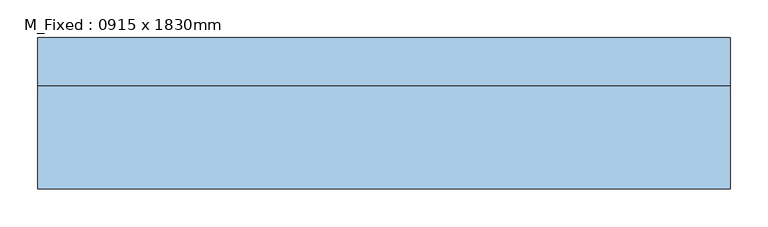
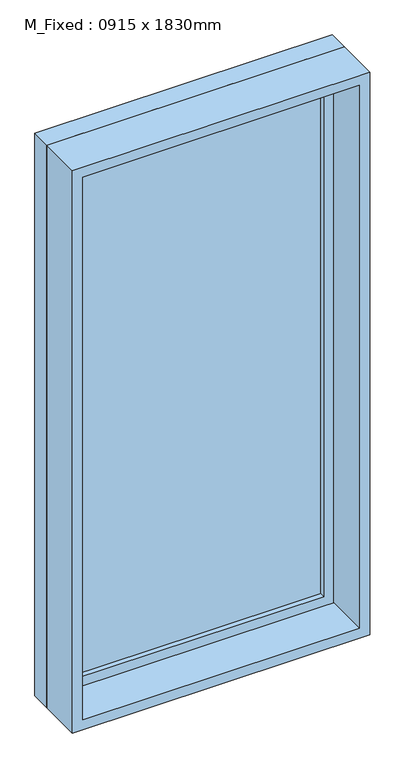
"""IFC4 building model written with IfcOpenShell, lengths in millimetres: window geometry, M_Fixed : 0915 x 1830mm."""

from ifc_helpers import new_model, si_unit, frame, origin, place, context, project, spatial, polyline, outline, extrude, source, transform, mapped, element, save


def m_fixed_0915_x_1830mm_5d6e8bc1(model_context):
    return source(origin(), model_context, "Body", "SweptSolid", [
        extrude(outline(polyline([(-394.5, 78.0), (394.5, 78.0), (394.5, 66.0), (-394.5, 66.0), (-394.5, 78.0)])), frame((0.0, 0.0, 368.0), z_axis=(0.0, 0.0, 1.0), x_axis=(1.0, 0.0, 0.0)), (0.0, 0.0, 1.0), 1704.0),
        extrude(outline(polyline([(2116.0, -438.5), (324.0, -438.5), (324.0, 438.5), (2116.0, 438.5), (2116.0, -438.5)]), holes=[polyline([(2072.0, -394.5), (2072.0, 394.5), (368.0, 394.5), (368.0, -394.5), (2072.0, -394.5)])]), frame((0.0, 50.0, 0.0), z_axis=(0.0, 1.0, 0.0), x_axis=(0.0, 0.0, 1.0)), (0.0, 0.0, 1.0), 44.0),
        extrude(outline(polyline([(2135.0, -457.5), (305.0, -457.5), (305.0, 457.5), (2135.0, 457.5), (2135.0, -457.5)]), holes=[polyline([(2116.0, -438.5), (2116.0, 438.5), (324.0, 438.5), (324.0, -438.5), (2116.0, -438.5)])]), frame((0.0, 50.0, 0.0), z_axis=(0.0, 1.0, 0.0), x_axis=(0.0, 0.0, 1.0)), (0.0, 0.0, 1.0), 63.0),
        extrude(outline(polyline([(2135.0, -457.5), (305.0, -457.5), (305.0, 457.5), (2135.0, 457.5), (2135.0, -457.5)]), holes=[polyline([(2103.0, -425.5), (2103.0, 425.5), (337.0, 425.5), (337.0, -425.5), (2103.0, -425.5)])]), frame((0.0, -87.0, 0.0), z_axis=(0.0, 1.0, 0.0), x_axis=(0.0, 0.0, 1.0)), (0.0, 0.0, 1.0), 137.0),
    ])


if __name__ == "__main__":
    model = new_model("IFC4")
    model_context = context("Model", 3, world=origin())
    ifc_project = project(units=[si_unit("LENGTHUNIT", "METRE", prefix="MILLI")], contexts=[model_context])
    site = spatial("IfcSite", under=ifc_project)
    building = spatial("IfcBuilding", under=site)
    placement = place(None, origin())
    m_fixed_0915_x_1830mm_shape = m_fixed_0915_x_1830mm_5d6e8bc1(model_context)
    element("IfcWindow", 1, ObjectType="M_Fixed : 0915 x 1830mm", at=placement, inside=building, context=model_context, shape_type="MappedRepresentation", body=[
        mapped(m_fixed_0915_x_1830mm_shape, transform((0.0, 0.0, 0.0), x_axis=(1.0, 0.0, 0.0), y_axis=(0.0, 1.0, 0.0), z_axis=(0.0, 0.0, 1.0))),
    ])
    save(model, "model.ifc")

# Revit data of these elements
# Type "M_Fixed : 0915 x 1830mm"
#   Type Mark = "18"
#   Height = 1830 mm
#   Default Sill Height = 305 mm
#   Width = 915 mm
#   Window Inset = 19 mm
#   Frame Exterior Material = Sash
#   Frame Interior Material = Sash
#   Glass Pane Material = Glass
#   Sash = Sash
#   Wall Closure = (empty or 0)
# Element 1 (IfcWindow, "M_Fixed : 0915 x 1830mm")
#   Materials on its faces: "Sash", "Glass"
# Materials
#   "Sash": class "Wood", colour RGB 136 99 55, transparency 0
#   "Glass": class "Glass", colour RGB 218 227 224, transparency 0.85, Description = "Soda Lime Glass", Cost = 0
